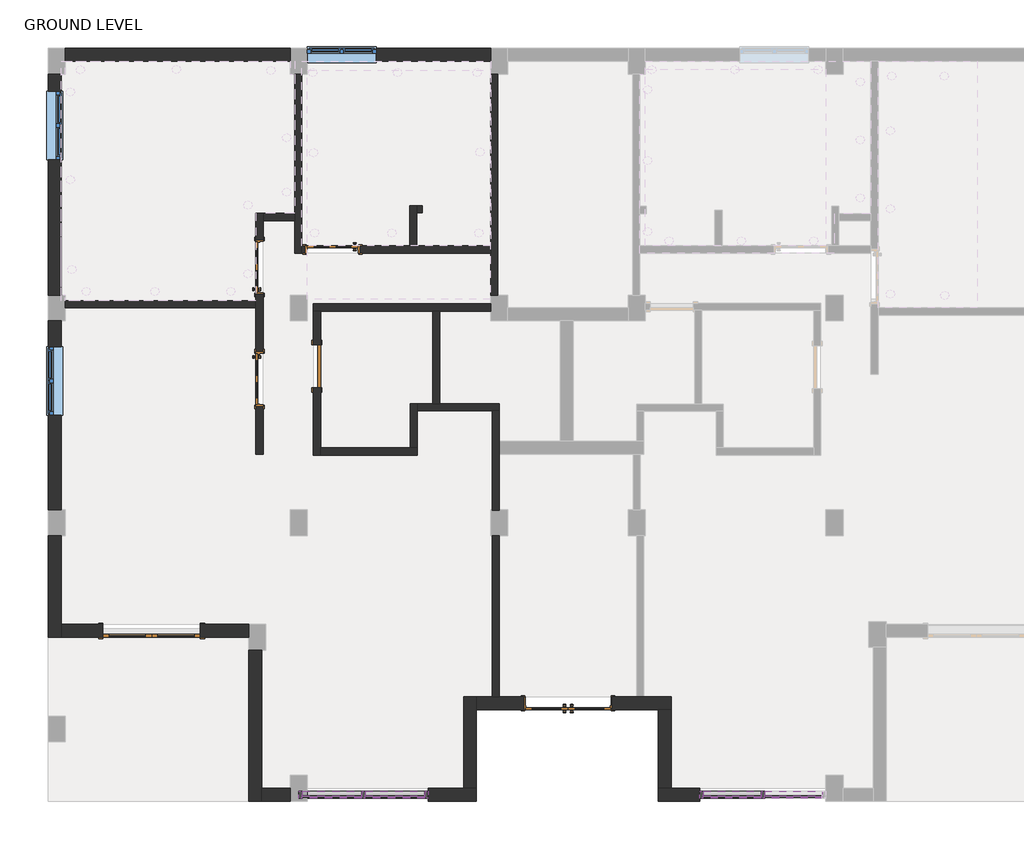
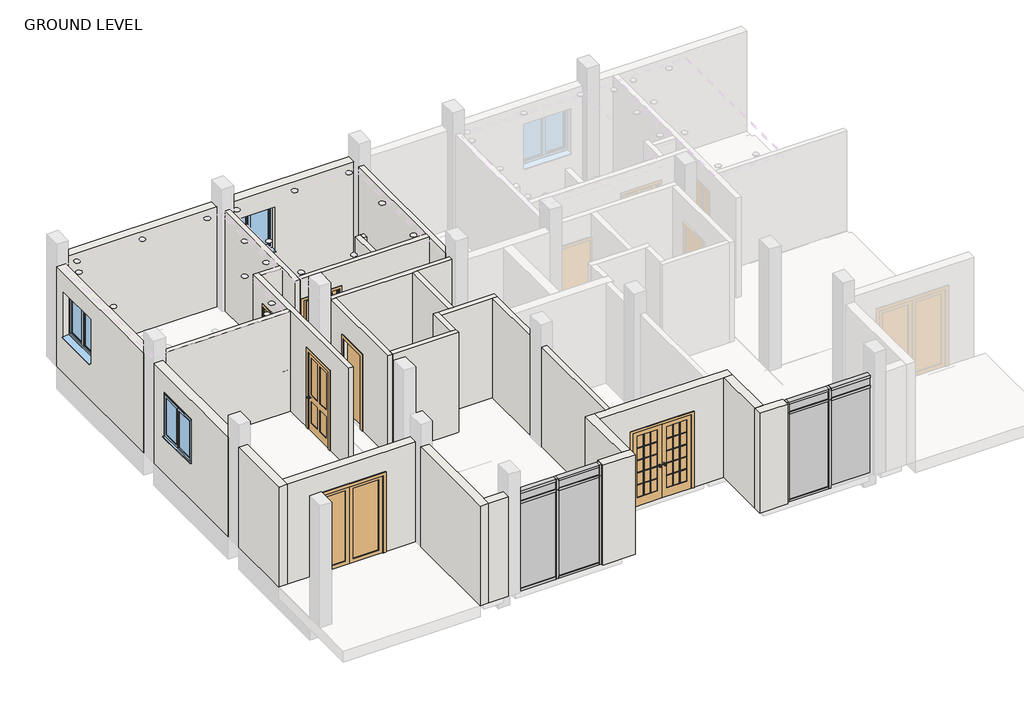
# One storey, part 1 of 5: 29 walls, 21 members, 8 plates, 6 doors, 3 windows.
"""IFC4 building model written with IfcOpenShell, lengths in millimetres."""

from ifc_helpers import new_model, si_unit, frame, origin, origin_with_axes, place, context, project, spatial, polyline, outline, extrude, faceted_brep, transform, mapped, element, save
from components import door_e52a3823, door_c5d3b7d7, door_68a706ac, door_a823658d, door_1fe7f57d, member_a1c24a98, member_38455fd9, member_f0fea5a5, member_ee409385, member_7fa39cca, member_afdd3af2, member_75d1e245, member_3c3dc66a, system_panel_glazed_958d1135, system_panel_glazed_0266aec6, system_panel_glazed_b341651b, system_panel_glazed_8433226c, w2_0001_windows_4_x_4_9dec5fc7

model = new_model("IFC4")

# Units and contexts
model_context = context("Model", 3, world=origin())
ifc_project = project(units=[si_unit("LENGTHUNIT", "METRE", prefix="MILLI")], contexts=[model_context])

# Site, building, storey
site = spatial("IfcSite", under=ifc_project)
building = spatial("IfcBuilding", under=site)
storey = spatial("IfcBuildingStorey", under=building, Name="GROUND LEVEL", Elevation=0.0)

# Doors
placement = place(None, origin())
door_shape = door_e52a3823(model_context)
element("IfcDoor", 1, ObjectType="Door-Double-Glass : 68\" x 84\"", at=placement, inside=storey, context=model_context, shape_type="MappedRepresentation", body=[
    mapped(door_shape, transform((-7309.9981098, -11554.5807833, 0.0), x_axis=(-1.0, 0.0, 0.0), y_axis=(0.0, -1.0, 0.0), z_axis=(0.0, 0.0, 1.0))),
])
door_2_shape = door_c5d3b7d7(model_context)
element("IfcDoor", 2, ObjectType="Door-Interior-Double-Full Glass-Wood : 60\" x 80\"", at=placement, inside=storey, context=model_context, shape_type="MappedRepresentation", body=[
    mapped(door_2_shape, transform((74.6824202, -12840.1152089, 0.0), x_axis=(-1.0, 0.0, 0.0), y_axis=(0.0, -1.0, 0.0), z_axis=(0.0, 0.0, 1.0))),
])
door_3_shape = door_68a706ac(model_context)
element("IfcDoor", 3, ObjectType="Door-Interior-Single-4_Panel-Wood : 36\" x 84\"", at=placement, inside=storey, context=model_context, shape_type="MappedRepresentation", body=[
    mapped(door_3_shape, transform((-5402.1925798, -5105.3620333, 0.0), x_axis=(0.0, 1.0, 0.0), y_axis=(-1.0, 0.0, 0.0), z_axis=(0.0, 0.0, 1.0))),
])
door_4_shape = door_a823658d(model_context)
element("IfcDoor", 4, ObjectType="Door-Interior-Single-4_Panel-Wood : 36\" x 84\"", at=placement, inside=storey, context=model_context, shape_type="MappedRepresentation", body=[
    mapped(door_4_shape, transform((-4103.6175798, -4789.1311634, 0.0), x_axis=(-1.0, 0.0, 0.0), y_axis=(0.0, -1.0, 0.0), z_axis=(0.0, 0.0, 1.0))),
])
element("IfcDoor", 5, ObjectType="Door-Interior-Single-4_Panel-Wood : 36\" x 84\"", at=placement, inside=storey, context=model_context, shape_type="MappedRepresentation", body=[
    mapped(door_4_shape, transform((-5402.1925798, -7092.9120333, 0.0), x_axis=(0.0, -1.0, 0.0), y_axis=(1.0, 0.0, 0.0), z_axis=(0.0, 0.0, 1.0))),
])
door_5_shape = door_1fe7f57d(model_context)
element("IfcDoor", 6, ObjectType="Single-Flush : 30\" x 80\"", at=placement, inside=storey, context=model_context, shape_type="MappedRepresentation", body=[
    mapped(door_5_shape, transform((-4379.0950401, -6863.7942903, 0.0), x_axis=(0.0, -1.0, 0.0), y_axis=(1.0, 0.0, 0.0), z_axis=(0.0, 0.0, 1.0))),
])

# Members
member_shape = member_a1c24a98(model_context)
element("IfcMember", 7, ObjectType="Rectangular Mullion : 2.5\" x 5\" rectangular", at=placement, inside=storey, context=model_context, shape_type="MappedRepresentation", body=[
    mapped(member_shape, transform((2474.9824202, -14462.5402089, 2743.2), x_axis=(0.0, 0.0, 1.0), y_axis=(0.0, 1.0, 0.0), z_axis=(-1.0, 0.0, 0.0))),
])
element("IfcMember", 8, ObjectType="Rectangular Mullion : 2.5\" x 5\" rectangular", at=placement, inside=storey, context=model_context, shape_type="MappedRepresentation", body=[
    mapped(member_shape, transform((3560.8324202, -14462.5402089, 2743.2), x_axis=(0.0, 0.0, 1.0), y_axis=(0.0, 1.0, 0.0), z_axis=(-1.0, 0.0, 0.0))),
])
element("IfcMember", 9, ObjectType="Rectangular Mullion : 2.5\" x 5\" rectangular", at=placement, inside=storey, context=model_context, shape_type="MappedRepresentation", body=[
    mapped(member_shape, transform((3497.3324202, -14462.5402089, 0.0), x_axis=(0.0, 0.0, -1.0), y_axis=(0.0, 1.0, 0.0), z_axis=(1.0, 0.0, 0.0))),
])
member_2_shape = member_38455fd9(model_context)
element("IfcMember", 10, ObjectType="Rectangular Mullion : 2.5\" x 5\" rectangular", at=placement, inside=storey, context=model_context, shape_type="MappedRepresentation", body=[
    mapped(member_2_shape, transform((3560.8324202, -14462.5402089, 2438.4), x_axis=(0.0, 0.0, 1.0), y_axis=(0.0, 1.0, 0.0), z_axis=(-1.0, 0.0, 0.0))),
])
element("IfcMember", 11, ObjectType="Rectangular Mullion : 2.5\" x 5\" rectangular", at=placement, inside=storey, context=model_context, shape_type="MappedRepresentation", body=[
    mapped(member_2_shape, transform((2474.9824202, -14462.5402089, 2438.4), x_axis=(0.0, 0.0, 1.0), y_axis=(0.0, 1.0, 0.0), z_axis=(-1.0, 0.0, 0.0))),
])
member_3_shape = member_f0fea5a5(model_context)
element("IfcMember", 12, ObjectType="Rectangular Mullion : 2.5\" x 5\" rectangular", at=placement, inside=storey, context=model_context, shape_type="MappedRepresentation", body=[
    mapped(member_3_shape, transform((3529.0824202, -14462.5402089, 0.0), x_axis=(-1.0, 0.0, 0.0), y_axis=(0.0, 1.0, 0.0), z_axis=(0.0, 0.0, -1.0))),
])
element("IfcMember", 13, ObjectType="Rectangular Mullion : 2.5\" x 5\" rectangular", at=placement, inside=storey, context=model_context, shape_type="MappedRepresentation", body=[
    mapped(member_3_shape, transform((-3551.1675798, -14462.5402089, 0.0), x_axis=(-1.0, 0.0, 0.0), y_axis=(0.0, 1.0, 0.0), z_axis=(0.0, 0.0, -1.0))),
])
member_4_shape = member_ee409385(model_context)
element("IfcMember", 14, ObjectType="Rectangular Mullion : 2.5\" x 5\" rectangular", at=placement, inside=storey, context=model_context, shape_type="MappedRepresentation", body=[
    mapped(member_4_shape, transform((2411.4824202, -14462.5402089, 0.0), x_axis=(-1.0, 0.0, 0.0), y_axis=(0.0, 1.0, 0.0), z_axis=(0.0, 0.0, -1.0))),
])
element("IfcMember", 15, ObjectType="Rectangular Mullion : 2.5\" x 5\" rectangular", at=placement, inside=storey, context=model_context, shape_type="MappedRepresentation", body=[
    mapped(member_4_shape, transform((-4700.5175798, -14462.5402089, 0.0), x_axis=(-1.0, 0.0, 0.0), y_axis=(0.0, 1.0, 0.0), z_axis=(0.0, 0.0, -1.0))),
])
element("IfcMember", 16, ObjectType="Rectangular Mullion : 2.5\" x 5\" rectangular", at=placement, inside=storey, context=model_context, shape_type="MappedRepresentation", body=[
    mapped(member_4_shape, transform((-2401.8175798, -14462.5402089, 2438.4), x_axis=(1.0, 0.0, 0.0), y_axis=(0.0, 1.0, 0.0), z_axis=(0.0, 0.0, 1.0))),
])
member_5_shape = member_7fa39cca(model_context)
element("IfcMember", 17, ObjectType="Rectangular Mullion : 2.5\" x 5\" rectangular", at=placement, inside=storey, context=model_context, shape_type="MappedRepresentation", body=[
    mapped(member_5_shape, transform((-4637.0175798, -14462.5402089, 2743.2), x_axis=(0.0, 0.0, 1.0), y_axis=(0.0, 1.0, 0.0), z_axis=(-1.0, 0.0, 0.0))),
])
element("IfcMember", 18, ObjectType="Rectangular Mullion : 2.5\" x 5\" rectangular", at=placement, inside=storey, context=model_context, shape_type="MappedRepresentation", body=[
    mapped(member_5_shape, transform((-3519.4175798, -14462.5402089, 2743.2), x_axis=(0.0, 0.0, 1.0), y_axis=(0.0, 1.0, 0.0), z_axis=(-1.0, 0.0, 0.0))),
])
element("IfcMember", 19, ObjectType="Rectangular Mullion : 2.5\" x 5\" rectangular", at=placement, inside=storey, context=model_context, shape_type="MappedRepresentation", body=[
    mapped(member_5_shape, transform((-2465.3175798, -14462.5402089, 0.0), x_axis=(0.0, 0.0, -1.0), y_axis=(0.0, 1.0, 0.0), z_axis=(1.0, 0.0, 0.0))),
])
element("IfcMember", 20, ObjectType="Rectangular Mullion : 2.5\" x 5\" rectangular", at=placement, inside=storey, context=model_context, shape_type="MappedRepresentation", body=[
    mapped(member_5_shape, transform((-3582.9175798, -14462.5402089, 0.0), x_axis=(0.0, 0.0, -1.0), y_axis=(0.0, 1.0, 0.0), z_axis=(1.0, 0.0, 0.0))),
])
member_6_shape = member_afdd3af2(model_context)
element("IfcMember", 21, ObjectType="Rectangular Mullion : 2.5\" x 5\" rectangular", at=placement, inside=storey, context=model_context, shape_type="MappedRepresentation", body=[
    mapped(member_6_shape, transform((-3519.4175798, -14462.5402089, 2438.4), x_axis=(0.0, 0.0, 1.0), y_axis=(0.0, 1.0, 0.0), z_axis=(-1.0, 0.0, 0.0))),
])
element("IfcMember", 22, ObjectType="Rectangular Mullion : 2.5\" x 5\" rectangular", at=placement, inside=storey, context=model_context, shape_type="MappedRepresentation", body=[
    mapped(member_6_shape, transform((-4637.0175798, -14462.5402089, 2438.4), x_axis=(0.0, 0.0, 1.0), y_axis=(0.0, 1.0, 0.0), z_axis=(-1.0, 0.0, 0.0))),
])
member_7_shape = member_75d1e245(model_context)
element("IfcMember", 23, ObjectType="Rectangular Mullion : 2.5\" x 5\" rectangular", at=placement, inside=storey, context=model_context, shape_type="MappedRepresentation", body=[
    mapped(member_7_shape, transform((3529.0824202, -14462.5402089, 2438.4), x_axis=(-1.0, 0.0, 0.0), y_axis=(0.0, 1.0, 0.0), z_axis=(0.0, 0.0, -1.0))),
])
element("IfcMember", 24, ObjectType="Rectangular Mullion : 2.5\" x 5\" rectangular", at=placement, inside=storey, context=model_context, shape_type="MappedRepresentation", body=[
    mapped(member_7_shape, transform((-3551.1675798, -14462.5402089, 2438.4), x_axis=(-1.0, 0.0, 0.0), y_axis=(0.0, 1.0, 0.0), z_axis=(0.0, 0.0, -1.0))),
])
member_8_shape = member_3c3dc66a(model_context)
element("IfcMember", 25, ObjectType="Rectangular Mullion : 2.5\" x 5\" rectangular", at=placement, inside=storey, context=model_context, shape_type="MappedRepresentation", body=[
    mapped(member_8_shape, transform((2411.4824202, -14462.5402089, 2438.4), x_axis=(-1.0, 0.0, 0.0), y_axis=(0.0, 1.0, 0.0), z_axis=(0.0, 0.0, -1.0))),
])
element("IfcMember", 26, ObjectType="Rectangular Mullion : 2.5\" x 5\" rectangular", at=placement, inside=storey, context=model_context, shape_type="MappedRepresentation", body=[
    mapped(member_8_shape, transform((-4700.5175798, -14462.5402089, 2438.4), x_axis=(-1.0, 0.0, 0.0), y_axis=(0.0, 1.0, 0.0), z_axis=(0.0, 0.0, -1.0))),
])
element("IfcMember", 27, ObjectType="Rectangular Mullion : 2.5\" x 5\" rectangular", at=placement, inside=storey, context=model_context, shape_type="MappedRepresentation", body=[
    mapped(member_8_shape, transform((-2401.8175798, -14462.5402089, 2743.2), x_axis=(1.0, 0.0, 0.0), y_axis=(0.0, 1.0, 0.0), z_axis=(0.0, 0.0, 1.0))),
])

# Plates
system_panel_glazed_shape = system_panel_glazed_958d1135(model_context)
element("IfcPlate", 28, ObjectType="System Panel : Glazed", at=placement, inside=storey, context=model_context, shape_type="MappedRepresentation", body=[
    mapped(system_panel_glazed_shape, transform((4072.0074202, -14462.5402089, 63.5), x_axis=(-1.0, 0.0, 0.0), y_axis=(0.0, -1.0, 0.0), z_axis=(0.0, 0.0, 1.0))),
])
element("IfcPlate", 29, ObjectType="System Panel : Glazed", at=placement, inside=storey, context=model_context, shape_type="MappedRepresentation", body=[
    mapped(system_panel_glazed_shape, transform((2986.1574202, -14462.5402089, 63.5), x_axis=(-1.0, 0.0, 0.0), y_axis=(0.0, -1.0, 0.0), z_axis=(0.0, 0.0, 1.0))),
])
system_panel_glazed_2_shape = system_panel_glazed_0266aec6(model_context)
element("IfcPlate", 30, ObjectType="System Panel : Glazed", at=placement, inside=storey, context=model_context, shape_type="MappedRepresentation", body=[
    mapped(system_panel_glazed_2_shape, transform((-2992.3675798, -14462.5402089, 63.5), x_axis=(-1.0, 0.0, 0.0), y_axis=(0.0, -1.0, 0.0), z_axis=(0.0, 0.0, 1.0))),
])
element("IfcPlate", 31, ObjectType="System Panel : Glazed", at=placement, inside=storey, context=model_context, shape_type="MappedRepresentation", body=[
    mapped(system_panel_glazed_2_shape, transform((-4109.9675798, -14462.5402089, 63.5), x_axis=(-1.0, 0.0, 0.0), y_axis=(0.0, -1.0, 0.0), z_axis=(0.0, 0.0, 1.0))),
])
system_panel_glazed_3_shape = system_panel_glazed_b341651b(model_context)
element("IfcPlate", 32, ObjectType="System Panel : Glazed", at=placement, inside=storey, context=model_context, shape_type="MappedRepresentation", body=[
    mapped(system_panel_glazed_3_shape, transform((-2992.3675798, -14462.5402089, 2470.15), x_axis=(-1.0, 0.0, 0.0), y_axis=(0.0, -1.0, 0.0), z_axis=(0.0, 0.0, 1.0))),
])
element("IfcPlate", 33, ObjectType="System Panel : Glazed", at=placement, inside=storey, context=model_context, shape_type="MappedRepresentation", body=[
    mapped(system_panel_glazed_3_shape, transform((-4109.9675798, -14462.5402089, 2470.15), x_axis=(-1.0, 0.0, 0.0), y_axis=(0.0, -1.0, 0.0), z_axis=(0.0, 0.0, 1.0))),
])
system_panel_glazed_4_shape = system_panel_glazed_8433226c(model_context)
element("IfcPlate", 34, ObjectType="System Panel : Glazed", at=placement, inside=storey, context=model_context, shape_type="MappedRepresentation", body=[
    mapped(system_panel_glazed_4_shape, transform((4072.0074202, -14462.5402089, 2470.15), x_axis=(-1.0, 0.0, 0.0), y_axis=(0.0, -1.0, 0.0), z_axis=(0.0, 0.0, 1.0))),
])
element("IfcPlate", 35, ObjectType="System Panel : Glazed", at=placement, inside=storey, context=model_context, shape_type="MappedRepresentation", body=[
    mapped(system_panel_glazed_4_shape, transform((2986.1574202, -14462.5402089, 2470.15), x_axis=(-1.0, 0.0, 0.0), y_axis=(0.0, -1.0, 0.0), z_axis=(0.0, 0.0, 1.0))),
])

# Walls
element("IfcWall", 36, ObjectType="EXTERIOR WALL 9\"", at=placement, inside=storey, context=model_context, shape_type="SweptSolid", body=[
    extrude(outline(polyline([(-4852.9175798, -1452.2061634), (-8839.9786397, -1452.2061634), (-8839.9786397, -1223.6061634), (-4852.9175798, -1223.6061634), (-4852.9175798, -1452.2061634)])), origin_with_axes(), (0.0, 0.0, 1.0), 2743.2),
])
element("IfcWall", 37, ObjectType="EXTERIOR WALL 9\"", at=placement, inside=storey, context=model_context, shape_type="SweptSolid", body=[
    extrude(outline(polyline([(1000.0, -3328.9175798), (1000.0, -4548.1175798), (0.0, -4548.1175798), (0.0, -1296.9175798), (2743.2, -1296.9175798), (2743.2, -4548.1175798), (2219.2, -4548.1175798), (2219.2, -3328.9175798), (1000.0, -3328.9175798)])), frame((0.0, -1452.2061634, 0.0), z_axis=(0.0, 1.0, 0.0), x_axis=(0.0, 0.0, 1.0)), (0.0, 0.0, 1.0), 228.6),
])
element("IfcWall", 38, ObjectType="EXTERIOR WALL 9\"", at=placement, inside=storey, context=model_context, shape_type="SweptSolid", body=[
    extrude(outline(polyline([(-1680.8061634, 0.0), (-5600.6620333, 0.0), (-5600.6620333, 2743.2), (-1680.8061634, 2743.2), (-1680.8061634, 0.0)]), holes=[polyline([(-3204.8061634, 1000.0), (-1985.6061634, 1000.0), (-1985.6061634, 2219.2), (-3204.8061634, 2219.2), (-3204.8061634, 1000.0)])]), frame((-9144.7786397, 0.0, 0.0), z_axis=(1.0, 0.0, 0.0), x_axis=(0.0, 1.0, 0.0)), (0.0, 0.0, 1.0), 228.6),
])
element("IfcWall", 39, ObjectType="EXTERIOR WALL 9\"", at=placement, inside=storey, context=model_context, shape_type="SweptSolid", body=[
    extrude(outline(polyline([(-6057.8620333, 0.0), (-9410.6620333, 0.0), (-9410.6620333, 2743.2), (-6057.8620333, 2743.2), (-6057.8620333, 0.0)]), holes=[polyline([(-6515.0620333, 1000.0), (-6515.0620333, 2219.2), (-7734.2620333, 2219.2), (-7734.2620333, 1000.0), (-6515.0620333, 1000.0)])]), frame((-9144.7786397, 0.0, 0.0), z_axis=(1.0, 0.0, 0.0), x_axis=(0.0, 1.0, 0.0)), (0.0, 0.0, 1.0), 228.6),
])
element("IfcWall", 40, ObjectType="EXTERIOR WALL 9\"", at=placement, inside=storey, context=model_context, shape_type="Brep", body=[
    faceted_brep([(-9144.7786397, -9867.8620333, 0.0), (-9144.7786397, -11671.2620333, 0.0), (-9144.7786397, -11671.2620333, 2743.2), (-9144.7786397, -9867.8620333, 2743.2), (-8916.1786397, -9867.8620333, 0.0), (-8916.1786397, -9867.8620333, 2743.2), (-8916.1786397, -11442.6620333, 2743.2), (-8916.1786397, -11671.2620333, 2743.2), (-8916.1786397, -11671.2620333, 0.0), (-8916.1786397, -11442.6620333, 0.0)], [[[0, 1, 2, 3]], [[4, 5, 6, 7, 8, 9]], [[1, 0, 4, 9, 8]], [[3, 2, 7, 6, 5]], [[0, 3, 5, 4]], [[2, 1, 8, 7]]]),
])
element("IfcWall", 41, ObjectType="EXTERIOR WALL 9\"", at=placement, inside=storey, context=model_context, shape_type="SweptSolid", body=[
    extrude(outline(polyline([(2743.2, -5589.5175798), (2743.2, -8916.1786397), (0.0, -8916.1786397), (0.0, -8173.5981098), (2133.6, -8173.5981098), (2133.6, -6446.3981098), (0.0, -6446.3981098), (0.0, -5589.5175798), (2743.2, -5589.5175798)])), frame((0.0, -11671.2620333, 0.0), z_axis=(0.0, 1.0, 0.0), x_axis=(0.0, 0.0, 1.0)), (0.0, 0.0, 1.0), 228.6),
])
element("IfcWall", 42, ObjectType="EXTERIOR WALL 9\"", at=placement, inside=storey, context=model_context, shape_type="Brep", body=[
    faceted_brep([(-5589.5175798, -11899.8620333, 0.0), (-5589.5175798, -14576.8402089, 0.0), (-5589.5175798, -14576.8402089, 2743.2), (-5589.5175798, -11899.8620333, 2743.2), (-5360.9175798, -11899.8620333, 0.0), (-5360.9175798, -11899.8620333, 2743.2), (-5360.9175798, -14348.2402089, 2743.2), (-5360.9175798, -14576.8402089, 2743.2), (-5360.9175798, -14576.8402089, 0.0), (-5360.9175798, -14348.2402089, 0.0)], [[[0, 1, 2, 3]], [[4, 5, 6, 7, 8, 9]], [[1, 0, 4, 9, 8]], [[3, 2, 7, 6, 5]], [[0, 3, 5, 4]], [[2, 1, 8, 7]]]),
])
element("IfcWall", 43, ObjectType="EXTERIOR WALL 9\"", at=placement, inside=storey, context=model_context, shape_type="SweptSolid", body=[
    extrude(outline(polyline([(-5360.9175798, -14348.2402089), (-4852.9175798, -14348.2402089), (-4852.9175798, -14576.8402089), (-5360.9175798, -14576.8402089), (-5360.9175798, -14348.2402089)])), origin_with_axes(), (0.0, 0.0, 1.0), 2743.2),
])
element("IfcWall", 44, ObjectType="EXTERIOR WALL 9\"", at=placement, inside=storey, context=model_context, shape_type="Brep", body=[
    faceted_brep([(1674.8824202, -14348.2402089, 0.0), (1674.8824202, -14348.2402089, 2743.2), (1903.4824202, -14348.2402089, 2743.2), (2411.4824202, -14348.2402089, 2743.2), (2411.4824202, -14348.2402089, 0.0), (1903.4824202, -14348.2402089, 0.0), (1674.8824202, -14576.8402089, 2743.2), (1674.8824202, -14576.8402089, 0.0), (2411.4824202, -14576.8402089, 0.0), (2411.4824202, -14576.8402089, 2743.2)], [[[0, 1, 2, 3, 4, 5]], [[6, 7, 8, 9]], [[7, 0, 5, 4, 8]], [[1, 6, 9, 3, 2]], [[1, 0, 7, 6]], [[4, 3, 9, 8]]]),
])
element("IfcWall", 45, ObjectType="EXTERIOR WALL 9\"", at=placement, inside=storey, context=model_context, shape_type="Brep", body=[
    faceted_brep([(-1550.9175798, -14576.8402089, 0.0), (-1550.9175798, -14576.8402089, 2743.2), (-2401.8175798, -14576.8402089, 2743.2), (-2401.8175798, -14576.8402089, 0.0), (-1550.9175798, -14348.2402089, 2743.2), (-1550.9175798, -14348.2402089, 0.0), (-1779.5175798, -14348.2402089, 0.0), (-2401.8175798, -14348.2402089, 0.0), (-2401.8175798, -14348.2402089, 2743.2), (-1779.5175798, -14348.2402089, 2743.2)], [[[0, 1, 2, 3]], [[4, 5, 6, 7, 8, 9]], [[5, 0, 3, 7, 6]], [[1, 4, 9, 8, 2]], [[1, 0, 5, 4]], [[3, 2, 8, 7]]]),
])
element("IfcWall", 46, ObjectType="EXTERIOR WALL 9\"", at=placement, inside=storey, context=model_context, shape_type="Brep", body=[
    faceted_brep([(-1550.9175798, -14348.2402089, 0.0), (-1550.9175798, -12951.2402089, 0.0), (-1550.9175798, -12722.6402089, 0.0), (-1550.9175798, -12722.6402089, 2743.2), (-1550.9175798, -12951.2402089, 2743.2), (-1550.9175798, -14348.2402089, 2743.2), (-1779.5175798, -14348.2402089, 0.0), (-1779.5175798, -14348.2402089, 2743.2), (-1779.5175798, -12722.6402089, 2743.2), (-1779.5175798, -12722.6402089, 0.0)], [[[0, 1, 2, 3, 4, 5]], [[6, 7, 8, 9]], [[2, 1, 0, 6, 9]], [[5, 4, 3, 8, 7]], [[0, 5, 7, 6]], [[3, 2, 9, 8]]]),
])
element("IfcWall", 47, ObjectType="EXTERIOR WALL 9\"", at=placement, inside=storey, context=model_context, shape_type="Brep", body=[
    faceted_brep([(1903.4824202, -12951.2402089, 2743.2), (1674.8824202, -12951.2402089, 2743.2), (-1550.9175798, -12951.2402089, 2743.2), (-1550.9175798, -12951.2402089, 0.0), (-712.7175798, -12951.2402089, 0.0), (-712.7175798, -12951.2402089, 2057.4), (862.0824202, -12951.2402089, 2057.4), (862.0824202, -12951.2402089, 0.0), (1674.8824202, -12951.2402089, 0.0), (1903.4824202, -12951.2402089, 0.0), (-1550.9175798, -12722.6402089, 2743.2), (-1271.5175798, -12722.6402089, 2743.2), (-1144.5175798, -12722.6402089, 2743.2), (1293.8824202, -12722.6402089, 2743.2), (1420.8824202, -12722.6402089, 2743.2), (1903.4824202, -12722.6402089, 2743.2), (1903.4824202, -12722.6402089, 0.0), (1420.8824202, -12722.6402089, 0.0), (1293.8824202, -12722.6402089, 0.0), (862.0824202, -12722.6402089, 0.0), (862.0824202, -12722.6402089, 2057.4), (-712.7175798, -12722.6402089, 2057.4), (-712.7175798, -12722.6402089, 0.0), (-1144.5175798, -12722.6402089, 0.0), (-1271.5175798, -12722.6402089, 0.0), (-1550.9175798, -12722.6402089, 0.0)], [[[0, 1, 2, 3, 4, 5, 6, 7, 8, 9]], [[10, 11, 12, 13, 14, 15, 16, 17, 18, 19, 20, 21, 22, 23, 24, 25]], [[3, 25, 24, 23, 22, 4]], [[16, 9, 8, 7, 19, 18, 17]], [[2, 1, 0, 15, 14, 13, 12, 11, 10]], [[3, 2, 10, 25]], [[0, 9, 16, 15]], [[21, 5, 4, 22]], [[5, 21, 20, 6]], [[6, 20, 19, 7]]]),
])
element("IfcWall", 48, ObjectType="EXTERIOR WALL 9\"", at=placement, inside=storey, context=model_context, shape_type="SweptSolid", body=[
    extrude(outline(polyline([(1674.8824202, -14348.2402089), (1674.8824202, -12951.2402089), (1903.4824202, -12951.2402089), (1903.4824202, -14348.2402089), (1674.8824202, -14348.2402089)])), origin_with_axes(), (0.0, 0.0, 1.0), 2743.2),
])
element("IfcWall", 49, ObjectType="INTERIOR WALL 5\"", at=placement, inside=storey, context=model_context, shape_type="SweptSolid", body=[
    extrude(outline(polyline([(-5462.5175798, -5829.2620333), (-8839.9786397, -5829.2620333), (-8839.9786397, -5702.2620333), (-5462.5175798, -5702.2620333), (-5462.5175798, -5829.2620333)])), origin_with_axes(), (0.0, 0.0, 1.0), 2743.2),
])
element("IfcWall", 50, ObjectType="INTERIOR WALL 5\"", at=placement, inside=storey, context=model_context, shape_type="Brep", body=[
    faceted_brep([(-5462.5175798, -8420.0620333, 0.0), (-5462.5175798, -8420.0620333, 2743.2), (-5462.5175798, -5829.2620333, 2743.2), (-5462.5175798, -5702.2620333, 2743.2), (-5462.5175798, -4153.3104011, 2743.2), (-5462.5175798, -4153.3104011, 0.0), (-5462.5175798, -4622.7620333, 0.0), (-5462.5175798, -4622.7620333, 2159.0), (-5462.5175798, -5587.9620333, 2159.0), (-5462.5175798, -5587.9620333, 0.0), (-5462.5175798, -5702.2620333, 0.0), (-5462.5175798, -5829.2620333, 0.0), (-5462.5175798, -6610.3120333, 0.0), (-5462.5175798, -6610.3120333, 2159.0), (-5462.5175798, -7575.5120333, 2159.0), (-5462.5175798, -7575.5120333, 0.0), (-5335.5175798, -8420.0620333, 2743.2), (-5335.5175798, -8420.0620333, 0.0), (-5335.5175798, -7575.5120333, 0.0), (-5335.5175798, -7575.5120333, 2159.0), (-5335.5175798, -6610.3120333, 2159.0), (-5335.5175798, -6610.3120333, 0.0), (-5335.5175798, -5587.9620333, 0.0), (-5335.5175798, -5587.9620333, 2159.0), (-5335.5175798, -4622.7620333, 2159.0), (-5335.5175798, -4622.7620333, 0.0), (-5335.5175798, -4280.3104011, 0.0), (-5335.5175798, -4153.3104011, 0.0), (-5335.5175798, -4153.3104011, 2743.2), (-5335.5175798, -4280.3104011, 2743.2)], [[[0, 1, 2, 3, 4, 5, 6, 7, 8, 9, 10, 11, 12, 13, 14, 15]], [[16, 17, 18, 19, 20, 21, 22, 23, 24, 25, 26, 27, 28, 29]], [[17, 0, 15, 18]], [[5, 27, 26, 25, 6]], [[9, 22, 21, 12, 11, 10]], [[1, 0, 17, 16]], [[4, 3, 2, 1, 16, 29, 28]], [[5, 4, 28, 27]], [[24, 7, 6, 25]], [[7, 24, 23, 8]], [[8, 23, 22, 9]], [[14, 19, 18, 15]], [[19, 14, 13, 20]], [[20, 13, 12, 21]]]),
])
element("IfcWall", 51, ObjectType="INTERIOR WALL 5\"", at=placement, inside=storey, context=model_context, shape_type="SweptSolid", body=[
    extrude(outline(polyline([(-4776.7175798, -4280.3104011), (-5335.5175798, -4280.3104011), (-5335.5175798, -4153.3104011), (-4776.7175798, -4153.3104011), (-4776.7175798, -4280.3104011)])), origin_with_axes(), (0.0, 0.0, 1.0), 2743.2),
])
element("IfcWall", 52, ObjectType="INTERIOR WALL 5\"", at=placement, inside=storey, context=model_context, shape_type="Brep", body=[
    faceted_brep([(-4776.7175798, -1680.8061634, 0.0), (-4776.7175798, -4153.3104011, 0.0), (-4776.7175798, -4280.3104011, 0.0), (-4776.7175798, -4855.8061634, 0.0), (-4776.7175798, -4855.8061634, 2743.2), (-4776.7175798, -4280.3104011, 2743.2), (-4776.7175798, -4153.3104011, 2743.2), (-4776.7175798, -1680.8061634, 2743.2), (-4649.7175798, -1680.8061634, 0.0), (-4649.7175798, -1680.8061634, 2743.2), (-4649.7175798, -4728.8061634, 2743.2), (-4649.7175798, -4855.8061634, 2743.2), (-4649.7175798, -4855.8061634, 0.0), (-4649.7175798, -4728.8061634, 0.0)], [[[0, 1, 2, 3, 4, 5, 6, 7]], [[8, 9, 10, 11, 12, 13]], [[3, 2, 1, 0, 8, 13, 12]], [[7, 6, 5, 4, 11, 10, 9]], [[0, 7, 9, 8]], [[4, 3, 12, 11]]]),
])
element("IfcWall", 53, ObjectType="INTERIOR WALL 5\"", at=placement, inside=storey, context=model_context, shape_type="Brep", body=[
    faceted_brep([(-1296.9175798, -4855.8061634, 2743.2), (-4649.7175798, -4855.8061634, 2743.2), (-4649.7175798, -4855.8061634, 0.0), (-4586.2175798, -4855.8061634, 0.0), (-4586.2175798, -4855.8061634, 2159.0), (-3621.0175798, -4855.8061634, 2159.0), (-3621.0175798, -4855.8061634, 0.0), (-1296.9175798, -4855.8061634, 0.0), (-4649.7175798, -4728.8061634, 2743.2), (-2732.0175798, -4728.8061634, 2743.2), (-2605.0175798, -4728.8061634, 2743.2), (-1296.9175798, -4728.8061634, 2743.2), (-1296.9175798, -4728.8061634, 0.0), (-2605.0175798, -4728.8061634, 0.0), (-2732.0175798, -4728.8061634, 0.0), (-3621.0175798, -4728.8061634, 0.0), (-3621.0175798, -4728.8061634, 2159.0), (-4586.2175798, -4728.8061634, 2159.0), (-4586.2175798, -4728.8061634, 0.0), (-4649.7175798, -4728.8061634, 0.0)], [[[0, 1, 2, 3, 4, 5, 6, 7]], [[8, 9, 10, 11, 12, 13, 14, 15, 16, 17, 18, 19]], [[2, 19, 18, 3]], [[12, 7, 6, 15, 14, 13]], [[1, 0, 11, 10, 9, 8]], [[2, 1, 8, 19]], [[0, 7, 12, 11]], [[17, 4, 3, 18]], [[4, 17, 16, 5]], [[5, 16, 15, 6]]]),
])
element("IfcWall", 54, ObjectType="INTERIOR WALL 5\"", at=placement, inside=storey, context=model_context, shape_type="Brep", body=[
    faceted_brep([(-1296.9175798, -1680.8061634, 0.0), (-1296.9175798, -4728.8061634, 0.0), (-1296.9175798, -4855.8061634, 0.0), (-1296.9175798, -5600.6620333, 0.0), (-1296.9175798, -5600.6620333, 2743.2), (-1296.9175798, -4855.8061634, 2743.2), (-1296.9175798, -4728.8061634, 2743.2), (-1296.9175798, -1680.8061634, 2743.2), (-1169.9175798, -1680.8061634, 0.0), (-1169.9175798, -1680.8061634, 2743.2), (-1169.9175798, -5600.6620333, 2743.2), (-1169.9175798, -5600.6620333, 0.0)], [[[0, 1, 2, 3, 4, 5, 6, 7]], [[8, 9, 10, 11]], [[3, 2, 1, 0, 8, 11]], [[4, 3, 11, 10]], [[7, 6, 5, 4, 10, 9]], [[0, 7, 9, 8]]]),
])
element("IfcWall", 55, ObjectType="INTERIOR WALL 5\"", at=placement, inside=storey, context=model_context, shape_type="Brep", body=[
    faceted_brep([(-2605.0175798, -4728.8061634, 0.0), (-2605.0175798, -4144.6061634, 0.0), (-2605.0175798, -4017.6061634, 0.0), (-2605.0175798, -4017.6061634, 2743.2), (-2605.0175798, -4144.6061634, 2743.2), (-2605.0175798, -4728.8061634, 2743.2), (-2732.0175798, -4728.8061634, 0.0), (-2732.0175798, -4728.8061634, 2743.2), (-2732.0175798, -4017.6061634, 2743.2), (-2732.0175798, -4017.6061634, 0.0)], [[[0, 1, 2, 3, 4, 5]], [[6, 7, 8, 9]], [[2, 1, 0, 6, 9]], [[5, 4, 3, 8, 7]], [[0, 5, 7, 6]], [[3, 2, 9, 8]]]),
])
element("IfcWall", 56, ObjectType="INTERIOR WALL 5\"", at=placement, inside=storey, context=model_context, shape_type="SweptSolid", body=[
    extrude(outline(polyline([(-2605.0175798, -4017.6061634), (-2516.1175798, -4017.6061634), (-2516.1175798, -4144.6061634), (-2605.0175798, -4144.6061634), (-2605.0175798, -4017.6061634)])), origin_with_axes(), (0.0, 0.0, 1.0), 2743.2),
])
element("IfcWall", 57, ObjectType="INTERIOR WALL 5\"", at=placement, inside=storey, context=model_context, shape_type="Brep", body=[
    faceted_brep([(-4442.5950401, -5885.8942903, 0.0), (-4315.5950401, -5885.8942903, 0.0), (-2325.6175798, -5885.8942903, 0.0), (-2198.6175798, -5885.8942903, 0.0), (-1296.9175798, -5885.8942903, 0.0), (-1296.9175798, -5885.8942903, 2743.2), (-2198.6175798, -5885.8942903, 2743.2), (-2325.6175798, -5885.8942903, 2743.2), (-4315.5950401, -5885.8942903, 2743.2), (-4442.5950401, -5885.8942903, 2743.2), (-4442.5950401, -5758.8942903, 0.0), (-4442.5950401, -5758.8942903, 2743.2), (-1296.9175798, -5758.8942903, 2743.2), (-1296.9175798, -5758.8942903, 0.0)], [[[0, 1, 2, 3, 4, 5, 6, 7, 8, 9]], [[10, 11, 12, 13]], [[4, 3, 2, 1, 0, 10, 13]], [[5, 4, 13, 12]], [[9, 8, 7, 6, 5, 12, 11]], [[0, 9, 11, 10]]]),
])
element("IfcWall", 58, ObjectType="INTERIOR WALL 5\"", at=placement, inside=storey, context=model_context, shape_type="Brep", body=[
    faceted_brep([(-4442.5950401, -7244.7942903, 2032.0), (-4442.5950401, -7244.7942903, 0.0), (-4442.5950401, -8439.1120333, 0.0), (-4442.5950401, -8439.1120333, 2743.2), (-4442.5950401, -5885.8942903, 2743.2), (-4442.5950401, -5885.8942903, 0.0), (-4442.5950401, -6482.7942903, 0.0), (-4442.5950401, -6482.7942903, 2032.0), (-4315.5950401, -8439.1120333, 0.0), (-4315.5950401, -8312.1120333, 0.0), (-4315.5950401, -7244.7942903, 0.0), (-4315.5950401, -7244.7942903, 2032.0), (-4315.5950401, -6482.7942903, 2032.0), (-4315.5950401, -6482.7942903, 0.0), (-4315.5950401, -5885.8942903, 0.0), (-4315.5950401, -5885.8942903, 2743.2), (-4315.5950401, -8312.1120333, 2743.2), (-4315.5950401, -8439.1120333, 2743.2)], [[[0, 1, 2, 3, 4, 5, 6, 7]], [[8, 9, 10, 11, 12, 13, 14, 15, 16, 17]], [[6, 5, 14, 13]], [[2, 1, 10, 9, 8]], [[4, 3, 17, 16, 15]], [[5, 4, 15, 14]], [[3, 2, 8, 17]], [[11, 10, 1, 0]], [[12, 11, 0, 7]], [[13, 12, 7, 6]]]),
])
element("IfcWall", 59, ObjectType="INTERIOR WALL 5\"", at=placement, inside=storey, context=model_context, shape_type="Brep", body=[
    faceted_brep([(-4315.5950401, -8439.1120333, 0.0), (-2601.0950401, -8439.1120333, 0.0), (-2601.0950401, -8439.1120333, 2743.2), (-4315.5950401, -8439.1120333, 2743.2), (-4315.5950401, -8312.1120333, 0.0), (-4315.5950401, -8312.1120333, 2743.2), (-2728.0950401, -8312.1120333, 2743.2), (-2601.0950401, -8312.1120333, 2743.2), (-2601.0950401, -8312.1120333, 0.0), (-2728.0950401, -8312.1120333, 0.0)], [[[0, 1, 2, 3]], [[4, 5, 6, 7, 8, 9]], [[1, 0, 4, 9, 8]], [[3, 2, 7, 6, 5]], [[0, 3, 5, 4]], [[2, 1, 8, 7]]]),
])
element("IfcWall", 60, ObjectType="INTERIOR WALL 5\"", at=placement, inside=storey, context=model_context, shape_type="Brep", body=[
    faceted_brep([(-2601.0950401, -8312.1120333, 0.0), (-2601.0950401, -7651.7120333, 0.0), (-2601.0950401, -7524.7120333, 0.0), (-2601.0950401, -7524.7120333, 2743.2), (-2601.0950401, -7651.7120333, 2743.2), (-2601.0950401, -8312.1120333, 2743.2), (-2728.0950401, -8312.1120333, 0.0), (-2728.0950401, -8312.1120333, 2743.2), (-2728.0950401, -7524.7120333, 2743.2), (-2728.0950401, -7524.7120333, 0.0)], [[[0, 1, 2, 3, 4, 5]], [[6, 7, 8, 9]], [[2, 1, 0, 6, 9]], [[5, 4, 3, 8, 7]], [[0, 5, 7, 6]], [[3, 2, 9, 8]]]),
])
element("IfcWall", 61, ObjectType="INTERIOR WALL 5\"", at=placement, inside=storey, context=model_context, shape_type="Brep", body=[
    faceted_brep([(-2601.0950401, -7651.7120333, 0.0), (-1271.5175798, -7651.7120333, 0.0), (-1144.5175798, -7651.7120333, 0.0), (-1144.5175798, -7651.7120333, 2743.2), (-1271.5175798, -7651.7120333, 2743.2), (-2601.0950401, -7651.7120333, 2743.2), (-2601.0950401, -7524.7120333, 0.0), (-2601.0950401, -7524.7120333, 2743.2), (-2325.6175798, -7524.7120333, 2743.2), (-2198.6175798, -7524.7120333, 2743.2), (-1144.5175798, -7524.7120333, 2743.2), (-1144.5175798, -7524.7120333, 0.0), (-2198.6175798, -7524.7120333, 0.0), (-2325.6175798, -7524.7120333, 0.0)], [[[0, 1, 2, 3, 4, 5]], [[6, 7, 8, 9, 10, 11, 12, 13]], [[2, 1, 0, 6, 13, 12, 11]], [[5, 4, 3, 10, 9, 8, 7]], [[0, 5, 7, 6]], [[3, 2, 11, 10]]]),
])
element("IfcWall", 62, ObjectType="INTERIOR WALL 5\"", at=placement, inside=storey, context=model_context, shape_type="SweptSolid", body=[
    extrude(outline(polyline([(-2325.6175798, -7524.7120333), (-2325.6175798, -5885.8942903), (-2198.6175798, -5885.8942903), (-2198.6175798, -7524.7120333), (-2325.6175798, -7524.7120333)])), origin_with_axes(), (0.0, 0.0, 1.0), 2743.2),
])
element("IfcWall", 63, ObjectType="INTERIOR WALL 5\"", at=placement, inside=storey, context=model_context, shape_type="Brep", body=[
    faceted_brep([(-1271.5175798, -7651.7120333, 0.0), (-1271.5175798, -9417.0120333, 0.0), (-1271.5175798, -9417.0120333, 2743.2), (-1271.5175798, -7651.7120333, 2743.2), (-1144.5175798, -7651.7120333, 0.0), (-1144.5175798, -7651.7120333, 2743.2), (-1144.5175798, -8197.8120333, 2743.2), (-1144.5175798, -8426.4120333, 2743.2), (-1144.5175798, -9417.0120333, 2743.2), (-1144.5175798, -9417.0120333, 0.0), (-1144.5175798, -8426.4120333, 0.0), (-1144.5175798, -8197.8120333, 0.0)], [[[0, 1, 2, 3]], [[4, 5, 6, 7, 8, 9, 10, 11]], [[1, 0, 4, 11, 10, 9]], [[2, 1, 9, 8]], [[3, 2, 8, 7, 6, 5]], [[0, 3, 5, 4]]]),
])
element("IfcWall", 64, ObjectType="INTERIOR WALL 5\"", at=placement, inside=storey, context=model_context, shape_type="SweptSolid", body=[
    extrude(outline(polyline([(-1271.5175798, -12722.6402089), (-1271.5175798, -9867.8620333), (-1144.5175798, -9867.8620333), (-1144.5175798, -12722.6402089), (-1271.5175798, -12722.6402089)])), origin_with_axes(), (0.0, 0.0, 1.0), 2743.2),
])

# Windows
w2_0001_windows_4_x_4_shape = w2_0001_windows_4_x_4_9dec5fc7(model_context)
element("IfcWindow", 65, ObjectType="w2.0001 : WINDOWS 4' X 4'", at=placement, inside=storey, context=model_context, shape_type="MappedRepresentation", body=[
    mapped(w2_0001_windows_4_x_4_shape, transform((-9030.4786397, -2595.2061634, 0.0), x_axis=(0.0, 1.0, 0.0), y_axis=(-1.0, 0.0, 0.0), z_axis=(0.0, 0.0, 1.0))),
])
element("IfcWindow", 66, ObjectType="w2.0001 : WINDOWS 4' X 4'", at=placement, inside=storey, context=model_context, shape_type="MappedRepresentation", body=[
    mapped(w2_0001_windows_4_x_4_shape, transform((-9030.4786397, -7124.6620333, 0.0), x_axis=(0.0, -1.0, 0.0), y_axis=(1.0, 0.0, 0.0), z_axis=(0.0, 0.0, 1.0))),
])
element("IfcWindow", 67, ObjectType="w2.0001 : WINDOWS 4' X 4'", at=placement, inside=storey, context=model_context, shape_type="MappedRepresentation", body=[
    mapped(w2_0001_windows_4_x_4_shape, transform((-3938.5175798, -1337.9061634, 0.0), x_axis=(-1.0, 0.0, 0.0), y_axis=(0.0, -1.0, 0.0), z_axis=(0.0, 0.0, 1.0))),
])

save(model, "model.ifc")

# Revit data of these elements
# Type "Door-Double-Glass : 68\" x 84\""
#   Type Mark = "11"
#   Construction Type Id = "opn-d45"
#   Assembly Code = "C1020"
#   Analytic Construction = "Wood frame, double glass door "
#   W = 2' - 10"
#   Thickness = 0' - 2"
#   Thermal Resistance (R) = 1.8150 (h·ft²·°F)/BTU
#   Swing Angle [instance default] = 90.00°
#   Heat Transfer Coefficient (U) = 0.5510 BTU/(h·ft²·°F)
#   Height = 7' - 0"
#   Bottom Rail = 0' - 4"
#   Top Rail = 0' - 4"
#   Stiles = 0' - 4"
#   Trim Projection = 0' - 1"
#   Trim Width = 0' - 3"
#   Width = 5' - 8"
#   Define Thermal Properties by = 1
#   Glazing = Glass
#   Panel Material = Wood - Birch - Solid Stained Light Low Gloss
#   Trim Material = Paint - Sienna
#   Visual Light Transmittance = 0
#   Solar Heat Gain Coefficient = 0
#   Function = (empty or 0)
#   Wall Closure = (empty or 0)
# Type "Door-Interior-Double-Full Glass-Wood : 60\" x 80\""
#   Type Mark = "8"
#   Assembly Code = "C1020300"
#   Analytic Construction = "French door, wood frame with single glass"
#   Top Rail = 0' - 4 11/16"
#   Thickness = 0' - 1 3/8"
#   Thermal Resistance (R) = 1.0696 (h·ft²·°F)/BTU
#   Swing Angle [instance default] = 90.00°
#   Stiles = 0' - 4 3/4"
#   Rough Width = 5' - 2"
#   Rough Height = 6' - 9"
#   Panel Width = 2' - 6"
#   Height = 6' - 8"
#   Width = 5' - 0"
#   Heat Transfer Coefficient (U) = 0.9350 BTU/(h·ft²·°F)
#   Bottom Rail = 0' - 9 1/8"
#   Show Grill [instance default] = yes
#   Trim Material = Cherry
#   Panel Material = Cherry
#   Frame Material = Cherry
#   Door Handle Material = Aluminum
#   Visual Light Transmittance = 0
#   Solar Heat Gain Coefficient = 0
#   Wall Closure = (empty or 0)
#   Function = (empty or 0)
# Type "Door-Interior-Single-4_Panel-Wood : 36\" x 84\""
#   Type Mark = "9"
#   Assembly Code = "C1020300"
#   Analytic Construction = "Wooden"
#   Top Rail = 0' - 4 11/16"
#   Thickness = 0' - 1 3/8"
#   Thermal Resistance (R) = 2.5876 (h·ft²·°F)/BTU
#   Swing Angle [instance default] = 90.00°
#   Stiles = 0' - 4 3/4"
#   Rough Width = 3' - 2"
#   Rough Height = 7' - 1"
#   Mullion = 0' - 4 1/2"
#   Lock Rail = 0' - 7 1/2"
#   Height = 7' - 0"
#   Width = 3' - 0"
#   Heat Transfer Coefficient (U) = 0.3865 BTU/(h·ft²·°F)
#   Bottom Rail = 0' - 9 1/8"
#   Trim Material = Cherry
#   Panel Material = Cherry
#   Frame Material = Cherry
#   Door Handle Material = Aluminum
#   Visual Light Transmittance = 0
#   Solar Heat Gain Coefficient = 0
#   Wall Closure = (empty or 0)
#   Function = (empty or 0)
# Type "Single-Flush : 30\" x 80\""
#   Type Mark = "5"
#   Construction Type Id = "MDOOR"
#   Assembly Code = "C1020"
#   Analytic Construction = "Metal"
#   Thickness = 0' - 2"
#   Heat Transfer Coefficient (U) = 0.651978 BTU/(h·ft²·°F)
#   Height = 6' - 8"
#   Trim Projection Ext = 0' - 1"
#   Trim Projection Int = 0' - 1"
#   Trim Width = 0' - 3"
#   Width = 2' - 6"
#   Define Thermal Properties by = 1
#   Define Thermal Properties by = 1
#   Door Material = Door - Panel
#   Frame Material = Door - Frame
#   Visual Light Transmittance = 0
#   Solar Heat Gain Coefficient = 0
#   Function = (empty or 0)
#   Wall Closure = (empty or 0)
# Type "Rectangular Mullion : 2.5\" x 5\" rectangular"
#   built-in parameter 1007304 = 0.416667 (stored number, unit not read)
#   built-in parameter 1007301 = 0.104167 (stored number, unit not read)
#   built-in parameter 1007300 = 0.104167 (stored number, unit not read)
# Type "System Panel : Glazed"
#   Construction Type Id = "GSP4R"
#   Analytic Construction = "1/8 in Pilkington single glazing"
#   Visual Light Transmittance = 0.9
#   Solar Heat Gain Coefficient = 0.86
#   Heat Transfer Coefficient (U) = 1.18115 BTU/(h·ft²·°F)
#   Define Thermal Properties by = 1
# Type "EXTERIOR WALL 9\""
#   Assembly Code = "B2010"
#   Layers, outside or top first: 0' - 9" "WARM BEIGE COLOUR" (function 1)
# Type "INTERIOR WALL 5\""
#   Assembly Code = "B2010"
#   Layers, outside or top first: 0' - 5" "WARM BEIGE COLOUR" (function 1)
# Type "w2.0001 : WINDOWS 4' X 4'"
#   Type Mark = "21"
#   Operation = "DoublePanelVertical"
#   Keynote = "16.05.01"
#   Analytic Construction = "<None>"
#   Rough Width = 4' - 0"
#   Rough Height = 4' - 0"
#   Rahmentiefe = 0' - 2.3622"
#   Rahmenhöhe unten = 0' - 3.14961"
#   Rahmehöhe oben = 0' - 3.14961"
#   Rahmenbreite = 0' - 2.3622"
#   Height = 4' - 0"
#   Flügeltiefe = 0' - 2.3622"
#   Flügelbreite = 0' - 2.3622"
#   Einbautiefe (von außen) [instance default] = 0' - 5.51181"
#   Width = 4' - 0"
#   Kippflügel [instance default] = yes
#   Drehflügel im Grundriß darstellen [instance default] = no
#   Drehflügel [instance default] = yes
#   Define Thermal Properties by = 1
#   Rahmen [instance default] = none
#   Glas [instance default] = none
#   Flügel [instance default] = none
#   Fensterbank aussen [instance default] = none
#   Fensterbank innen [instance default] = none
#   Wall Closure = (empty or 0)
# Element 1 (IfcDoor, "Door-Double-Glass : 68\" x 84\"")
#   Phase Created = New Construction
#   Materials on its faces: "Wood - Birch - Solid Stained Light Low Gloss", "Paint - Sienna", "Glass"
# Element 2 (IfcDoor, "Door-Interior-Double-Full Glass-Wood : 60\" x 80\"")
#   Swing Angle = 90.00°
#   Show Grill = yes
#   Phase Created = New Construction
#   Materials on its faces: "Cherry", "Aluminum", "Glass"
# Elements 3, 4, 5 (IfcDoor, "Door-Interior-Single-4_Panel-Wood : 36\" x 84\"")
#   Swing Angle = 90.00°
#   Phase Created = New Construction
#   Materials on its faces: "Cherry", "Aluminum"
# Element 6 (IfcDoor, "Single-Flush : 30\" x 80\"")
#   Phase Created = New Construction
#   Materials on its faces: "Door - Frame", "Door - Panel"
# Elements 7, 8, 9, 10, 11, 12, 13, 14, 15, 16, 17, 18, 19, 20, 21, 22, 23, 24, 25, 26, 27 (IfcMember, "Rectangular Mullion : 2.5\" x 5\" rectangular")
#   Phase Created = New Construction
#   Materials on its faces: "Aluminum"
# Elements 28, 29, 30, 31, 32, 33, 34, 35 (IfcPlate, "System Panel : Glazed")
#   Phase Created = New Construction
#   Materials on its faces: "Glass"
# Elements 36, 37, 38, 39, 40, 41, 42, 43, 44, 45, 46, 47, 48 (IfcWall, "EXTERIOR WALL 9\"")
#   Top Offset = -2' - 0"
#   Base Offset = 0' - 0"
#   wall height = 9' - 0"
#   Phase Created = New Construction
#   Base Constraint = GROUND LEVEL
#   Top Constraint = FIRST FLR
#   Materials on its faces: "WARM BEIGE COLOUR"
# Elements 49, 50, 51, 52, 53, 54, 55, 56, 57, 58, 59, 60, 61, 62, 63, 64 (IfcWall, "INTERIOR WALL 5\"")
#   Top Offset = -2' - 0"
#   Base Offset = 0' - 0"
#   wall height = 9' - 0"
#   Phase Created = New Construction
#   Base Constraint = GROUND LEVEL
#   Top Constraint = FIRST FLR
#   Materials on its faces: "WARM BEIGE COLOUR"
# Element 65 (IfcWindow, "w2.0001 : WINDOWS 4' X 4'")
#   Mark = "3"
#   Einbautiefe (von außen) = 0' - 5.51181"
#   Kippflügel = yes
#   Drehflügel im Grundriß darstellen = no
#   Drehflügel = yes
#   Rahmen = none
#   Glas = none
#   Flügel = none
#   Fensterbank innen = none
#   Fensterbank aussen = none
#   Phase Created = New Construction
#   Materials on its faces: "Fenster - Kunststoff", "Fenster - Kunststoff weiss", "Glass", "Fenster - Holz"
# Element 66 (IfcWindow, "w2.0001 : WINDOWS 4' X 4'")
#   Mark = "4"
#   Einbautiefe (von außen) = 0' - 5.51181"
#   Kippflügel = yes
#   Drehflügel im Grundriß darstellen = no
#   Drehflügel = yes
#   Rahmen = none
#   Glas = none
#   Flügel = none
#   Fensterbank innen = none
#   Fensterbank aussen = none
#   Phase Created = New Construction
#   Materials on its faces: "Fenster - Kunststoff", "Fenster - Kunststoff weiss", "Glass", "Fenster - Holz"
# Element 67 (IfcWindow, "w2.0001 : WINDOWS 4' X 4'")
#   Mark = "8"
#   Einbautiefe (von außen) = 0' - 5.51181"
#   Kippflügel = yes
#   Drehflügel im Grundriß darstellen = no
#   Drehflügel = yes
#   Rahmen = none
#   Glas = none
#   Flügel = none
#   Fensterbank innen = none
#   Fensterbank aussen = none
#   Phase Created = New Construction
#   Materials on its faces: "Fenster - Kunststoff", "Fenster - Kunststoff weiss", "Glass", "Fenster - Holz"
# Materials
#   "Glass": class "Glass", colour RGB 0 128 192, transparency 0.75, Description = "Soda Lime Glass", Cost = 0
#   "Wood - Birch - Solid Stained Light Low Gloss": class "Wood", colour RGB 210 159 95, transparency 0, Cost = 0
#   "Paint - Sienna": colour RGB 118 70 51, transparency 0, Cost = 0
#   "Cherry": class "Wood", colour RGB 226 177 128, transparency 0, Description = "Prunus Serotina", Cost = 0
#   "Aluminum": class "Metal", colour RGB 247 247 247, transparency 0, Description = "Aluminum 6061", Cost = 0
#   "Door - Panel": class "Wood", colour RGB 210 159 95, transparency 0, Cost = 0
#   "Door - Frame": colour RGB 118 70 51, transparency 0, Cost = 0
#   "WARM BEIGE COLOUR": class "Generic", colour RGB 120 120 120, transparency 0, Cost = 0
#   "Fenster - Kunststoff": colour RGB 249 249 249, transparency 0
#   "Fenster - Kunststoff weiss": colour RGB 249 249 249, transparency 0
#   "Fenster - Holz": colour RGB 216 135 75, transparency 0
# Room at (5161.032, -4506.556) mm, phase "New Construction", upper level "GROUND LEVEL", upper offset 10' - 0", lower offset 0' - 0"
#   Number = "1"
#   Name = "Room"
# Room at (-3320.606, -7099.003) mm, phase "New Construction", upper level "GROUND LEVEL", upper offset 10' - 0", lower offset 0' - 0"
#   Number = "2"
#   Name = "BATH"
# Room at (3440.182, -7093.569) mm, phase "New Construction", upper level "GROUND LEVEL", upper offset 10' - 0", lower offset 0' - 0"
#   Number = "3"
#   Name = "BATH"
# Room at (-2973.318, -3065.106) mm, phase "New Construction", upper level "GROUND LEVEL", upper offset 10' - 0", lower offset 0' - 0"
#   Number = "4"
#   Name = "BED ROOM"
# Room at (3395.732, -3065.106) mm, phase "New Construction", upper level "GROUND LEVEL", upper offset 10' - 0", lower offset 0' - 0"
#   Number = "5"
#   Name = "BED ROOM"
# Room at (7307.332, -3615.334) mm, phase "New Construction", upper level "GROUND LEVEL", upper offset 10' - 0", lower offset 0' - 0"
#   Number = "6"
#   Name = "BED ROOM"
# Room at (1217.682, -7061.491) mm, phase "New Construction", upper level "GROUND LEVEL", upper offset 10' - 0", lower offset 0' - 0"
#   Number = "7"
# Room at (23.882, -3640.734) mm, phase "New Construction", upper level "GROUND LEVEL", upper offset 10' - 0", lower offset 0' - 0"
#   Number = "8"
#   Name = "STAIRS"
# Room at (-1106.418, -7067.253) mm, phase "New Construction", upper level "GROUND LEVEL", upper offset 10' - 0", lower offset 0' - 0"
#   Number = "9"
# Room at (-6871.848, -3551.834) mm, phase "New Construction", upper level "GROUND LEVEL", upper offset 10' - 0", lower offset 0' - 0"
#   Number = "10"
#   Name = "BED ROOM"
# Room at (74.682, -10574.526) mm, phase "New Construction", upper level "GROUND LEVEL", upper offset 10' - 0", lower offset 0' - 0"
#   Number = "11"
#   Name = "STAIRS"
# Room at (-5119.248, -9339.675) mm, phase "New Construction", upper level "GROUND LEVEL", upper offset 10' - 0", lower offset 0' - 0"
#   Number = "12"
#   Name = "DINING AND KITCHEN"
# Room at (5192.782, -9627.423) mm, phase "New Construction", upper level "GROUND LEVEL", upper offset 10' - 0", lower offset 0' - 0"
#   Number = "13"
#   Name = "DINING AND KITCHEN"
